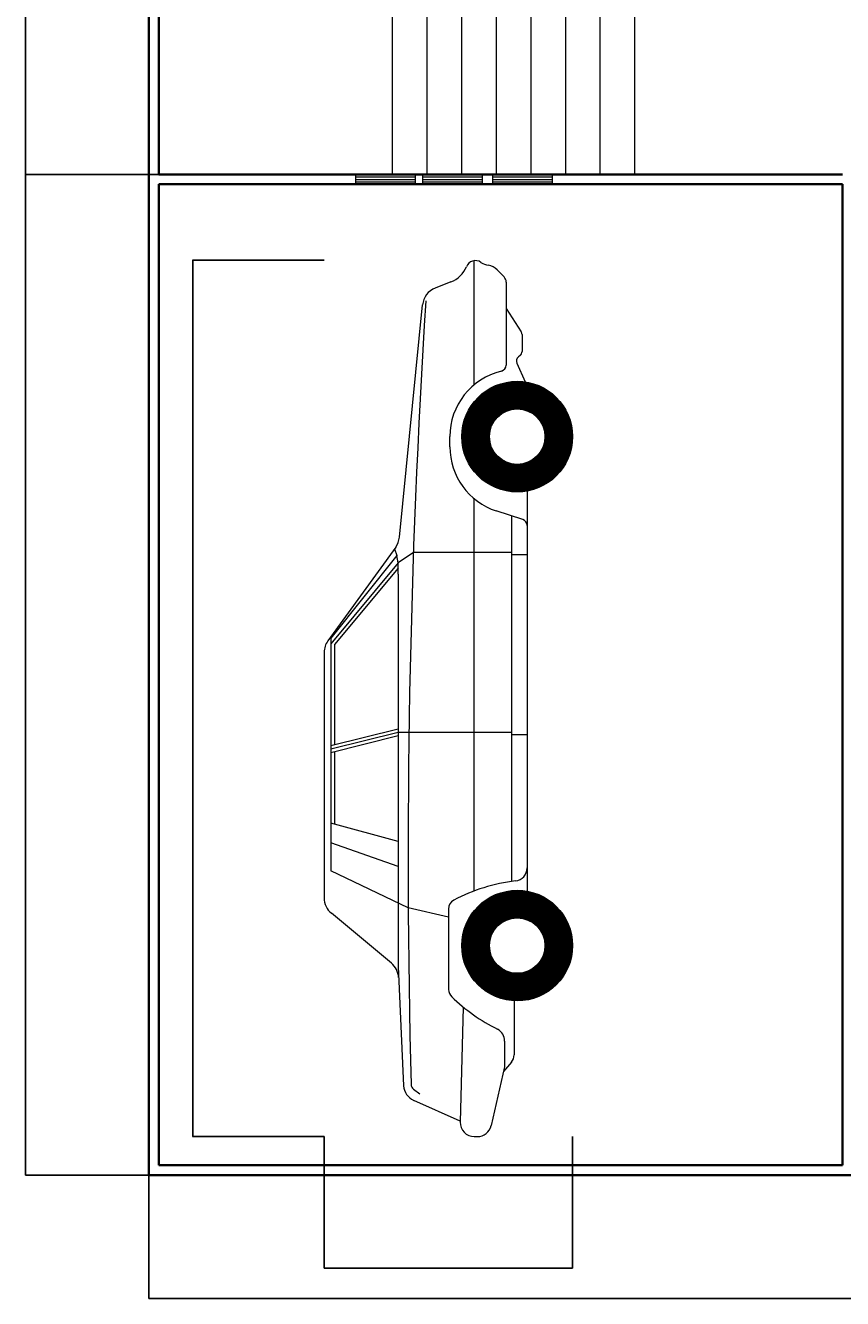
# Model space of a CAD drawing. Units: millimetres. Extents: x 1194 to 22780, y 83 to 13378.
# Tile 1 of 6: x 1194 to 5317, y 83 to 6507. Entities that reach past the tile are written whole.
import ezdxf

# ---------------------------------------------------------------- set-up
doc = ezdxf.new("R2010")
doc.units = ezdxf.units.MM
for name, color, linetype, lineweight in [('A-ANNO-DIMS', 2, 'Continuous', 18), ('A-FLOR-STRS', 7, 'Continuous', 18), ('A-GLAZ', 4, 'Continuous', 18), ('A-WALL', 7, 'Continuous', 35), ('C-PRKG-VEHI', 8, 'Continuous', 13)]:
    doc.layers.add(name, color=color, linetype=linetype, lineweight=lineweight)
doc.styles.get("Standard").update_dxf_attribs({"font": 'arial.ttf'})
doc.dimstyles.get("Standard").update_dxf_attribs({"dimtxt": 0.18, "dimasz": 0.18, "dimexe": 0.18, "dimexo": 0.0625, "dimgap": 0.09, "dimtad": 0, "dimtih": 1, "dimtoh": 1, "dimdec": 4, "dimzin": 0, "dimdsep": 46, "dimtxsty": 'Standard', "dimcen": 0.09, "dimadec": 0, "dimazin": 0, "dimtfac": 1, "dimtdec": 4, "dimtofl": 0, "dimtmove": 0, "dimatfit": 3, "dimfxl": 1, "dimtolj": 1, "dimtzin": 0, "dimarcsym": 0})

# ---------------------------------------------------------------- blocks, each defined once
blk = doc.blocks.new('Window - Wood Frame 36 in. Wide plan')
for p, q in [((0, 6), (0, 0)), ((0, 4.5), (36, 4.5)), ((0, 3), (36, 3)), ((0, 1.5), (36, 1.5)), ((36, 6), (36, 0))]:
    blk.add_line(p, q)
blk = doc.blocks.new('Car - sedan  side')
for p, q in [((-77.81068420410156, 49.34489536285401), (-126.5815277099609, 49.34489536285401)), ((-56.86628723144531, 35.13198184967041), (-75.48481750488281, 48.592209815979)), ((-139.5284881591797, 35.99398899078369), (-129.6360626220703, 47.91069889068603)), ((-128.5748443603515, 32.63923740386963), (-121.220962524414, 48.02381992340087)), ((-74.69862365722656, 48.02381992340087), (-121.220962524414, 48.02381992340087)), ((-120.3240203857422, 34.66572666168213), (-115.6691131591797, 48.02381992340087)), ((-115.3951263427734, 34.66572666168213), (-111.7413482666015, 48.02381992340087)), ((-97.54905700683592, 47.30442905426025), (-111.9381256103515, 47.30442905426025)), ((-94.41258239746094, 34.66572666168213), (-97.72758483886717, 48.02381992340087)), ((-93.7204132080078, 34.66572666168213), (-97.03541564941406, 48.02381992340087)), ((-93.02824401855469, 34.66572666168213), (-96.34324645996095, 48.02381992340087)), ((-76.25682067871092, 47.30442905426025), (-96.1647186279297, 47.30442905426025)), ((-61.08241271972656, 34.65577030181885), (-76.25682067871092, 47.30442905426025)), ((-60.02259826660156, 34.64692783355713), (-76.07066345214842, 48.02381992340087)), ((-58.53855895996094, 34.9260950088501), (-74.99412536621092, 48.02381992340087)), ((-140.2292327880859, 34.66572666168213), (-163.8789825439453, 33.55760288238526)), ((-62.27659606933594, 34.66572666168213), (-140.2292327880859, 34.66572666168213)), ((-93.7204132080078, 19.617600440979), (-93.7204132080078, 34.66572666168213)), ((-62.27659606933594, 34.66572666168213), (-60.02259826660156, 34.64692783355713)), ((-60.02259826660156, 34.64692783355713), (-58.53855895996094, 34.9260950088501)), ((-57.96794128417968, 31.6116189956665), (-60.02259826660156, 34.64692783355713)), ((-57.21324157714843, 35.38280582427979), (-58.53855895996094, 34.9260950088501)), ((-54.93388366699218, 34.39884281158447), (-8.750152587890625, 29.79911136627197)), ((-170.9268341064453, 22.322678565979), (-166.8111114501953, 31.55533695220948)), ((-164.5701141357422, 31.59879398345947), (-165.477066040039, 30.35254001617432)), ((-130.387466430664, 24.62635135650635), (-128.5748443603515, 32.63923740386963)), ((-57.96794128417968, 19.617600440979), (-57.96794128417968, 31.6116189956665)), ((-4.213516235351562, 24.18151950836182), (-5.418975830078125, 27.27166080474854)), ((-128.7820892333984, 24.62635135650635), (-144.7874603271484, 24.62635135650635)), ((-36.96612548828125, 24.38024997711182), (-34.94134521484375, 24.38024997711182)), ((-148.258804321289, 21.69713687896729), (-171.1068878173827, 22.32765293121338)), ((-173.9999847412109, 19.51329135894775), (-173.9999847412109, 18.90704441070556)), ((-47.20359802246093, 19.617600440979), (-125.2291412353516, 19.617600440979)), ((-93.7204132080078, 12.14150333404541), (-93.7204132080078, 19.617600440979)), ((-57.96794128417968, 12.14150333404541), (-57.96794128417968, 19.617600440979)), ((0, 19.617600440979), (-24.70387268066406, 19.617600440979)), ((-160.1240997314453, 13.48350620269775), (-171.8135528564453, 16.16277408599853)), ((-159.2159271240234, 12.14260196685791), (-161.0849456787109, 13.70372867584228)), ((-155.0106964111328, 13.48350620269775), (-160.1240997314453, 13.48350620269775)), ((-51.40187072753906, 9.887986183166502), (-49.69332885742187, 15.13794040679931)), ((-4.226425170898437, 13.18863773345947), (-20.72282409667969, 13.18863773345947)), ((-9.504730224609375, 13.18863773345947), (-14.09825134277344, 10.20021152496338)), ((-3.219284057617187, 13.59266757965088), (-1.773956298828125, 14.97469425201416)), ((-147.0265960693359, 11.60259342193603), (-157.7270355224609, 11.60259342193603)), ((-50.66848754882812, 12.14150333404541), (-123.3179779052734, 12.14150333404541)), ((-94.21171569824219, 9.029206275939941), (-94.21171569824219, 12.14150333404541)), ((-58.38966369628906, 9.029206275939941), (-58.38966369628906, 12.14150333404541)), ((-20.36183166503906, 11.06443881988525), (-24.05572509765625, 9.441704750061035)), ((-18.82789611816406, 10.41797733306885), (-19.11149597167969, 10.7644510269165)), ((-120.6163482666015, 9.029206275939941), (-125.2286224365234, 9.029206275939941)), ((-45.76005554199219, 9.029206275939941), (-120.6163482666015, 9.029206275939941)), ((-14.67802429199219, 10.02821445465088), (-18.00518798828125, 10.02821445465088))]:
    blk.add_line(p, q)
at = {"const_width": 5.48799991607666}
for points in [[(-127.7953033447265, 10.99602603912353, -0.9999999562886108), (-144.299331665039, 10.99602603912353, -0.9999999562886108)], [(-26.6893310546875, 10.99602603912353, -0.9999999562886108), (-43.193359375, 10.99602603912353, -0.9999999562886108)]]:
    blk.add_lwpolyline(points, format="xyb", close=True, dxfattribs=at)
for centre, radius in [((-136.0473175048828, 10.99602603912353), 10.99602603912353), ((-34.94134521484375, 10.99602603912353), 10.99602603912353), ((-136.0473175048828, 10.99602603912353), 5.508002281188964), ((-34.94134521484375, 10.99602603912353), 5.508002281188964)]:
    blk.add_circle(centre, radius)
for centre, radius, start, end in [((-126.5815277099609, 45.37503147125244), 3.969859600067138, 89.99999749552184, 140.3028756570888), ((-77.81068420410156, 45.37503147125244), 3.969859600067138, 54.1350361638109, 89.99999749552184), ((-142.5830535888672, 38.52964878082275), 3.969859600067138, 272.6826517359256, 320.3028808934163), ((-163.7206268310547, 30.17765903472901), 3.383651733398437, 92.68266357507108, 155.9736177264713), ((-54.54045104980469, 38.34915256500244), 3.969859600067138, 234.1350311548545, 264.3123095495883), ((-163.6219635009766, 30.90879917144775), 1.172623634338378, 91.49104828190312, 143.9552715044289), ((-118.5118255615234, -1702.123755455017), 1734.792114257812, 86.34698010096723, 91.49104828190312), ((-9.146713256835938, 25.81747531890869), 4.001329898834228, 21.31069063548193, 84.31230089816628), ((-118.093521118164, -2.781126976013183), 38.84752655029297, 136.3964001877188, 152.9097400063221), ((-144.7874603271484, 22.64237308502197), 1.983983039855957, 89.99999749552184, 136.3964001877188), ((-128.7820892333984, 22.64237308502197), 1.983983039855957, 28.1370958806946, 89.99999749552184), ((-157.1376495361328, 7.478318214416503), 34.13963699340821, 6.513536591134625, 28.1370958806946), ((-36.96612548828125, 10.99602603912353), 13.38422584533691, 89.99999749552184, 161.9731602707608), ((-34.94134521484375, 10.99602603912353), 13.38422584533691, 13.58641604273627, 89.99999749552184), ((0.9045410156250568, 26.17807102203369), 5.493702888488769, 201.3106992869039, 247.7048411864857), ((-171.1845550537109, 19.51329135894775), 2.815431356430053, 88.41927315552743, 180), ((-1.917068481445312, 19.29661655426025), 1.943759799003601, 325.3743646540424, 67.70484619544203), ((-171.1845550537109, 18.90704441070556), 2.815431356430053, 180, 257.0905319740804), ((2.457336425781193, 16.27603244781494), 3.372188329696654, 145.3743662479041, 172.3838635235148), ((-3.821029663085937, 17.1155481338501), 2.962058544158935, 313.7173490994733, 352.3838696136159), ((-155.0106964111328, 16.10243320465088), 2.618927478790283, 269.9999993167547, 332.9097435351022), ((-20.72282409667969, 14.43228244781494), 1.243641138076782, 193.5864110337799, 269.9999993167547), ((-4.226425170898437, 14.64594364166259), 1.457302808761596, 269.9999993167547, 313.7173490994733), ((-157.7270355224609, 13.92514896392822), 2.322556018829345, 230.1291252066421, 269.9999993167547), ((-120.6163482666015, 11.64813327789306), 2.618927478790283, 186.5135315821783, 269.9999993167547), ((-19.93421936035156, 10.09104251861572), 1.06317925453186, 39.3010264187021, 113.7159237656126), ((-18.00518798828125, 11.09139347076416), 1.06317925453186, 219.3010350701241, 269.9999993167547), ((-14.67802429199219, 11.09139347076416), 1.06317925453186, 269.9999993167547, 303.0469680308909), ((-52.58445739746093, 10.27285099029541), 1.243641138076782, 269.9999993167547, 341.9731586768991)]:
    blk.add_arc(centre, radius, start, end)
blk = doc.blocks.new('STAIR-DUPLEX-FLIGHT')
for p, q in [((1176.96885325314, 2725.862485348514), (1176.968853253142, -0.0001152583818111)), ((1351.817410696747, 2725.862485348514), (1351.817410696749, -0.0001152583818111)), ((1526.665968140353, 2725.862485348514), (1526.665968140356, -0.0001152583818111)), ((1701.514525583962, 2725.862485348514), (1701.514525583963, -0.0001152583818111)), ((1876.363083027568, 2725.862485348514), (1876.36308302757, -0.0001152583818111)), ((2051.211640471177, 2725.862485348514), (2051.211640471178, -0.0001152583818111)), ((2226.060197914782, 2725.862485348514), (2226.060197914785, -0.0001152583818111)), ((2400.908755358392, 2725.862485348514), (2400.908755358392, -0.0001152583818111)), ((1176.968853253141, 1562.931185045065), (0.0001000200393264, 1562.931185045065)), ((2400.908755358392, 1562.931185045066), (1176.968853253141, 1562.931185045065)), ((1186.968853253141, 1552.931185045065), (2390.908755358392, 1552.931185045065)), ((1186.968853253141, 1172.931185045065), (1186.968853253141, 1552.931185045064)), ((2390.908755358392, 1552.931185045065), (2390.908755358392, 1172.931185045064)), ((2400.908755358392, 1362.931185045066), (2400.908755358392, 1562.931185045066)), ((2400.908755358392, 1162.931185045065), (0.0001000200397812, 1162.931185045066)), ((2390.908755358392, 1172.931185045065), (1186.968853253141, 1172.931185045065))]:
    blk.add_line(p, q)
blk = doc.blocks.new('*D49')
at = {"layer": 'A-ANNO-DIMS', "color": 0, "lineweight": -2, "transparency": 16777216}
for p, q in [((2701.55068353055, 5322.648652153862), (2038.059772313744, 5322.648652153861)), ((2038.239772313744, 5322.468652153861), (2038.239772313745, 3111.587017674922)), ((2038.239772313745, 900.339244041822), (2038.239772313745, 3111.220878520761)), ((2701.550683530549, 900.1592440418221), (2038.059772313745, 900.1592440418219))]:
    blk.add_line(p, q, dxfattribs=at)
at = {"layer": 'A-ANNO-DIMS', "color": 0, "transparency": 16777216}
for points in [[(2038.209772313744, 5322.468652153861), (2038.269772313745, 5322.468652153861), (2038.239772313744, 5322.648652153861)], [(2038.209772313745, 900.339244041822), (2038.269772313745, 900.339244041822), (2038.239772313745, 900.1592440418219)]]:
    blk.add_solid(points, dxfattribs=at)
at = {"layer": 'Defpoints', "color": 0, "transparency": 16777216}
for p in [(2038.239772313744, 5322.648652153861), (2701.61318353055, 5322.648652153862), (2701.613183530549, 900.1592440418221)]:
    blk.add_point(p, dxfattribs=at)
at = {"layer": 'A-ANNO-DIMS', "color": 0, "transparency": 16777216, "insert": (2038.239772313745, 3111.403948097841), "char_height": 0.18, "attachment_point": 5}
blk.add_mtext('\\A1;SEDAN 4422', dxfattribs=at)
blk = doc.blocks.new('*D50')
at = {"layer": 'A-ANNO-DIMS', "color": 0, "lineweight": -2, "transparency": 16777216}
for p, q in [((2701.613183530549, 900.0967440418216), (2701.613183530549, 236.605832825016)), ((3954.97352574704, 900.0967440418216), (3954.97352574704, 236.605832825016)), ((2701.793183530548, 236.785832825016), (3327.943054502369, 236.785832825016)), ((3954.793525747041, 236.785832825016), (3328.64365477522, 236.785832825016))]:
    blk.add_line(p, q, dxfattribs=at)
at = {"layer": 'A-ANNO-DIMS', "color": 0, "transparency": 16777216}
for points in [[(2701.793183530548, 236.815832825016), (2701.793183530548, 236.755832825016), (2701.613183530549, 236.785832825016)], [(3954.793525747041, 236.815832825016), (3954.793525747041, 236.755832825016), (3954.97352574704, 236.785832825016)]]:
    blk.add_solid(points, dxfattribs=at)
at = {"layer": 'Defpoints', "color": 0, "transparency": 16777216}
for p in [(2701.613183530549, 900.1592440418217), (3954.97352574704, 900.1592440418217), (2701.613183530549, 236.785832825016)]:
    blk.add_point(p, dxfattribs=at)
at = {"layer": 'A-ANNO-DIMS', "color": 0, "transparency": 16777216, "insert": (3328.293354638794, 236.785832825016), "char_height": 0.18, "attachment_point": 5}
blk.add_mtext('\\A1;1253', dxfattribs=at)
blk = doc.blocks.new('*D51')
at = {"layer": 'A-ANNO-DIMS', "color": 0, "lineweight": -2, "transparency": 16777216}
for p, q in [((1817.4811, 705.711385), (1817.4811, 83.093885)), ((10867.4811, 705.711385), (10867.4811, 83.093885)), ((1817.6611, 83.273885), (6342.122634788541, 83.273885)), ((10867.3011, 83.273885), (6342.839565211459, 83.273885))]:
    blk.add_line(p, q, dxfattribs=at)
at = {"layer": 'A-ANNO-DIMS', "color": 0, "transparency": 16777216}
for points in [[(1817.6611, 83.30388500000001), (1817.6611, 83.243885), (1817.4811, 83.273885)], [(10867.3011, 83.30388500000001), (10867.3011, 83.243885), (10867.4811, 83.273885)]]:
    blk.add_solid(points, dxfattribs=at)
at = {"layer": 'Defpoints', "color": 0, "transparency": 16777216}
for p in [(1817.4811, 705.773885), (10867.4811, 705.773885), (10867.4811, 83.273885)]:
    blk.add_point(p, dxfattribs=at)
at = {"layer": 'A-ANNO-DIMS', "color": 0, "transparency": 16777216, "insert": (6342.4811, 83.273885), "char_height": 0.18, "attachment_point": 5}
blk.add_mtext('\\A1;9050', dxfattribs=at)
blk = doc.blocks.new('*D59')
at = {"layer": 'A-ANNO-DIMS', "color": 0, "lineweight": -2, "transparency": 16777216}
for p, q in [((1867.418600000001, 5755.773885000001), (1194.473081, 5755.773885000001)), ((1194.653081, 5755.593885000001), (1194.653081000001, 3230.955788137791)), ((1194.653081000001, 705.9538849999999), (1194.653081000001, 3230.591981862211)), ((1817.418600000001, 705.7738850000001), (1194.473081000001, 705.773885))]:
    blk.add_line(p, q, dxfattribs=at)
at = {"layer": 'A-ANNO-DIMS', "color": 0, "transparency": 16777216}
for points in [[(1194.623081, 5755.593885000001), (1194.683081, 5755.593885000001), (1194.653081, 5755.773885000001)], [(1194.623081000001, 705.9538849999999), (1194.683081000001, 705.9538849999999), (1194.653081000001, 705.773885)]]:
    blk.add_solid(points, dxfattribs=at)
at = {"layer": 'Defpoints', "color": 0, "transparency": 16777216}
for p in [(1194.653081, 5755.773885000001), (1867.481100000001, 5755.773885000001), (1817.481100000001, 705.7738850000001)]:
    blk.add_point(p, dxfattribs=at)
at = {"layer": 'A-ANNO-DIMS', "color": 0, "transparency": 16777216, "insert": (1194.653081000001, 3230.773885), "char_height": 0.18, "attachment_point": 5}
blk.add_mtext('\\A1;5050', dxfattribs=at)
blk = doc.blocks.new('*D60')
at = {"layer": 'A-ANNO-DIMS', "color": 0, "lineweight": -2, "transparency": 16777216}
for p, q in [((1867.418600000001, 8481.636485000005), (1194.473081000001, 8481.636485000005)), ((1194.653081, 8481.456485000004), (1194.653081000001, 7118.887088137793)), ((1194.653081000001, 5755.953885000002), (1194.653081000001, 7118.523281862214)), ((1867.418600000001, 5755.773885000001), (1194.473081000001, 5755.773885000001))]:
    blk.add_line(p, q, dxfattribs=at)
at = {"layer": 'A-ANNO-DIMS', "color": 0, "transparency": 16777216}
for points in [[(1194.623081, 8481.456485000004), (1194.683081, 8481.456485000004), (1194.653081, 8481.636485000005)], [(1194.623081000001, 5755.953885000002), (1194.683081000001, 5755.953885000002), (1194.653081000001, 5755.773885000001)]]:
    blk.add_solid(points, dxfattribs=at)
at = {"layer": 'Defpoints', "color": 0, "transparency": 16777216}
for p in [(1194.653081, 8481.636485000005), (1867.481100000001, 8481.636485000005), (1867.481100000001, 5755.773885000001)]:
    blk.add_point(p, dxfattribs=at)
at = {"layer": 'A-ANNO-DIMS', "color": 0, "transparency": 16777216, "insert": (1194.653081000002, 7118.705185000002), "char_height": 0.18, "attachment_point": 5}
blk.add_mtext('\\A1;2726', dxfattribs=at)

msp = doc.modelspace()

# ---------------------------------------------------------------- linework, layer by layer
at = {"layer": 'A-WALL'}
for p, q in [((1817.481100020039, 12730.77388474161), (1817.481100020041, 730.7738847416167)), ((1867.481100020039, 9505.773884741619), (1867.48110002004, 5755.773884741616)), ((4842.481100020041, 5755.773884741617), (1867.481100020039, 5755.773884741614)), ((4842.481100020041, 5755.773884741617), (5317.481100020039, 5755.773884741617)), ((4842.481100020041, 5705.773884741617), (1867.481100020039, 5705.773884741616)), ((1867.481100020039, 5705.773884741616), (1867.48110002004, 755.7738847416167)), ((4842.481100020041, 5705.773884741617), (5317.481100020038, 5705.773884741616)), ((5317.481100020039, 5705.773884741616), (5317.481100020039, 755.7738847416167)), ((1817.481100020041, 730.7738847416153), (1817.48110002004, 705.7738847416167)), ((1867.481100020041, 755.7738847416167), (5317.481100020039, 755.7738847416167)), ((1867.481100020041, 755.7738847416166), (4842.481100020041, 755.7738847416167)), ((1817.48110002004, 705.7738847416167), (1842.481100020041, 705.7738847416167)), ((1842.481100020041, 705.7738847416167), (5367.481100020039, 705.7738847416167)), ((1842.481100020041, 705.7738847416167), (4842.481100020041, 705.7738847416167))]:
    msp.add_line(p, q, dxfattribs=at)

# ---------------------------------------------------------------- block references
at = {"layer": 'A-FLOR-STRS'}
msp.add_blockref('STAIR-DUPLEX-FLIGHT', (1867.481, 5755.774), dxfattribs=at)
at = {"layer": 'A-GLAZ', "xscale": 8.388003104210137, "yscale": 8.388003104210137, "zscale": 8.388003104210137}
for p in [(2859.333539398887, 5705.445866116354), (3197.64405890304, 5705.445866116355), (3550.628066437377, 5705.445866116355)]:
    msp.add_blockref('Window - Wood Frame 36 in. Wide plan', p, dxfattribs=at)
at = {"layer": 'C-PRKG-VEHI', "xscale": 25.4, "yscale": 25.4, "zscale": 25.4, "rotation": 90}
msp.add_blockref('Car - sedan  side', (3954.97352574704, 5319.758898859402), dxfattribs=at)

# ---------------------------------------------------------------- dimensions: what is measured, and where the dimension line sits
at = {"layer": 'A-ANNO-DIMS'}
for base, p1, p2, angle, picture, middle in [((1194.653081, 8481.636485000005), (1867.4811, 5755.773884999999), (1867.4811, 8481.636485), 90, '*D60', (1194.653081000002, 7118.705185000002)), ((1194.653081, 5755.773885000001), (1817.4811, 705.773885), (1867.4811, 5755.773884999999), 90, '*D59', (1194.653081000001, 3230.773885)), ((2701.613183530549, 236.785832825016), (3954.97352574704, 900.1592440418217), (2701.613183530549, 900.1592440418217), 180, '*D50', (3328.293354638794, 236.785832825016))]:
    dim = msp.add_linear_dim(base=base, p1=p1, p2=p2, angle=angle, dimstyle='Standard', override={"dimdec": 0, "dimlfac": 1, "dimrnd": 0, "dimzin": 0, "dimdsep": 46, "dimlunit": 2}, dxfattribs=at)
    dim.commit()
    dim.dimension.update_dxf_attribs({"geometry": picture, "text_midpoint": middle})
dim = msp.add_linear_dim(base=(2038.239772313744, 5322.648652153861), p1=(2701.613183530549, 900.1592440418217), p2=(2701.613183530549, 5322.64865215386), angle=90, text='SEDAN <>', dimstyle='Standard', override={"dimdec": 0, "dimlfac": 1, "dimrnd": 0, "dimzin": 0, "dimdsep": 46, "dimlunit": 2}, dxfattribs=at)
dim.commit()
dim.dimension.update_dxf_attribs({"geometry": '*D49', "text_midpoint": (2038.239772313745, 3111.403948097841)})
dim = msp.add_linear_dim(base=(10867.4811, 83.273885), p1=(1817.4811, 705.773885), p2=(10867.4811, 705.773885), dimstyle='Standard', override={"dimdec": 0, "dimlfac": 1, "dimrnd": 0, "dimzin": 0, "dimdsep": 46, "dimlunit": 2}, dxfattribs=at)
dim.commit()
dim.dimension.update_dxf_attribs({"geometry": '*D51', "text_midpoint": (6342.4811, 83.273885)})

doc.saveas('drawing.dxf')
